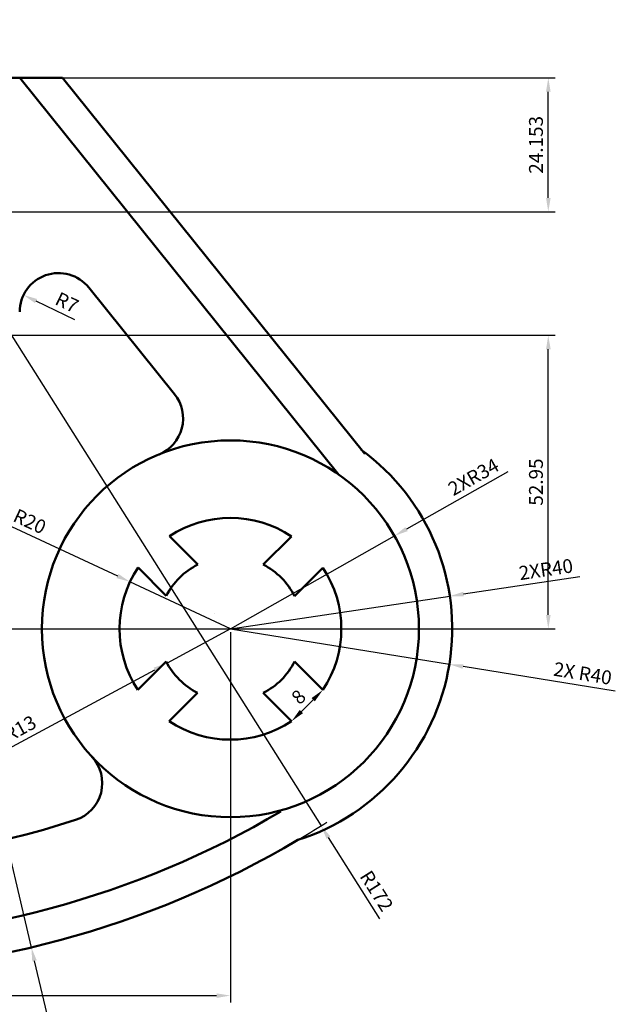
# Model space of a CAD drawing. Units: millimetres. Extents: x 2455 to 2735, y 1365 to 1648.
# Tile 3 of 3: x 2628 to 2735, y 1460 to 1637. Entities that reach past the tile are written whole.
import ezdxf

# ---------------------------------------------------------------- set-up
doc = ezdxf.new("R2010")
doc.units = ezdxf.units.MM
doc.linetypes.add('CENTER', pattern=[50.8, 31.75, -6.35, 6.35, -6.35])
for name, color, linetype, lineweight in [('M-CNTR', 4, 'CENTER', 18), ('M-CONS', 8, 'Continuous', 13), ('M-DIMS', 2, 'Continuous', 25), ('M-OUTL', 7, 'Continuous', 50)]:
    doc.layers.add(name, color=color, linetype=linetype, lineweight=lineweight)
doc.styles.get("Standard").update_dxf_attribs({"font": 'arial.ttf'})
doc.dimstyles.new('ISO-25', dxfattribs={"dimtxt": 2.5, "dimasz": 2.5, "dimexe": 1.25, "dimexo": 0.625, "dimtad": 1, "dimdec": 0, "dimtxsty": 'Standard', "dimcen": 2.5, "dimadec": 0, "dimazin": 0, "dimtfac": 1, "dimtdec": 0, "dimtmove": 0, "dimatfit": 3, "dimfxl": 1, "dimarcsym": 0})

# ---------------------------------------------------------------- blocks, each defined once
blk = doc.blocks.new('*D6')
at = {"layer": 'Defpoints', "color": 0, "transparency": 16777216}
for p in [(2515.88, 1527.3), (2665.87, 1527.3), (2665.87, 1461.12)]:
    blk.add_point(p, dxfattribs=at)
at = {"layer": 'M-DIMS', "color": 0, "lineweight": -2, "transparency": 16777216}
for p, q in [((2515.88, 1526.68), (2515.88, 1459.87)), ((2665.87, 1526.68), (2665.87, 1459.87)), ((2518.38, 1461.12), (2663.37, 1461.12))]:
    blk.add_line(p, q, dxfattribs=at)
at = {"layer": 'M-DIMS', "color": 0, "transparency": 16777216}
for points in [[(2518.38, 1461.53), (2518.38, 1460.7), (2515.88, 1461.12)], [(2663.37, 1461.53), (2663.37, 1460.7), (2665.87, 1461.12)]]:
    blk.add_solid(points, dxfattribs=at)
at = {"layer": 'M-DIMS', "color": 0, "transparency": 16777216, "insert": (2590.87, 1463.02), "char_height": 2.5, "attachment_point": 5}
blk.add_mtext('150', dxfattribs=at)
blk = doc.blocks.new('*D13')
at = {"layer": 'Defpoints', "color": 0, "transparency": 16777216}
for p in [(2628.57, 1587.53), (2634.88, 1584.49)]:
    blk.add_point(p, dxfattribs=at)
at = {"layer": 'M-DIMS', "color": 0, "lineweight": -2, "transparency": 16777216}
blk.add_line((2637.83, 1583.07), (2630.82, 1586.44), dxfattribs=at)
at = {"layer": 'M-DIMS', "color": 0, "transparency": 16777216}
blk.add_solid([(2631, 1586.82), (2630.64, 1586.07), (2628.57, 1587.53)], dxfattribs=at)
at = {"layer": 'M-DIMS', "color": 0, "transparency": 16777216, "insert": (2636.27, 1585.9), "char_height": 2.5, "attachment_point": 5, "rotation": 334.2857}
blk.add_mtext('R7', dxfattribs=at)
blk = doc.blocks.new('*D16')
at = {"layer": 'Defpoints', "color": 0, "transparency": 16777216}
for p in [(2647.76, 1535.78), (2665.88, 1527.3)]:
    blk.add_point(p, dxfattribs=at)
at = {"layer": 'M-DIMS', "color": 0, "lineweight": -2, "transparency": 16777216}
for p, q in [((2625.49, 1546.19), (2645.49, 1536.84)), ((2665.88, 1527.3), (2647.76, 1535.78))]:
    blk.add_line(p, q, dxfattribs=at)
at = {"layer": 'M-DIMS', "color": 0, "transparency": 16777216}
blk.add_solid([(2645.67, 1537.21), (2645.32, 1536.46), (2647.76, 1535.78)], dxfattribs=at)
at = {"layer": 'M-DIMS', "color": 0, "transparency": 16777216, "insert": (2629.56, 1546.39), "char_height": 2.5, "attachment_point": 5, "rotation": 334.9373}
blk.add_mtext('R20', dxfattribs=at)
blk = doc.blocks.new('*D17')
at = {"layer": 'Defpoints', "color": 0, "transparency": 16777216}
for p in [(2665.88, 1527.3), (2654.44, 1521.12)]:
    blk.add_point(p, dxfattribs=at)
at = {"layer": 'M-DIMS', "color": 0, "lineweight": -2, "transparency": 16777216}
for p, q in [((2665.88, 1527.3), (2654.44, 1521.12)), ((2625.82, 1505.64), (2652.24, 1519.93))]:
    blk.add_line(p, q, dxfattribs=at)
at = {"layer": 'M-DIMS', "color": 0, "transparency": 16777216}
blk.add_solid([(2652.04, 1520.3), (2652.44, 1519.56), (2654.44, 1521.12)], dxfattribs=at)
at = {"layer": 'M-DIMS', "color": 0, "transparency": 16777216, "insert": (2628.09, 1509.03), "char_height": 2.5, "attachment_point": 5, "rotation": 28.4115}
blk.add_mtext('R13', dxfattribs=at)
blk = doc.blocks.new('*D20')
at = {"layer": 'Defpoints', "color": 0, "transparency": 16777216}
for p in [(2695.46, 1544.07), (2665.88, 1527.3)]:
    blk.add_point(p, dxfattribs=at)
at = {"layer": 'M-DIMS', "color": 0, "lineweight": -2, "transparency": 16777216}
for p, q in [((2715.88, 1555.64), (2697.63, 1545.3)), ((2665.88, 1527.3), (2695.46, 1544.07))]:
    blk.add_line(p, q, dxfattribs=at)
at = {"layer": 'M-DIMS', "color": 0, "transparency": 16777216}
blk.add_solid([(2697.43, 1545.66), (2697.84, 1544.93), (2695.46, 1544.07)], dxfattribs=at)
at = {"layer": 'M-DIMS', "color": 0, "transparency": 16777216, "insert": (2709.87, 1554.42), "char_height": 2.5, "attachment_point": 5, "rotation": 29.5354}
blk.add_mtext('2XR34', dxfattribs=at)
blk = doc.blocks.new('*D21')
at = {"layer": 'Defpoints', "color": 0, "transparency": 16777216}
for p in [(2705.44, 1533.2), (2665.88, 1527.3)]:
    blk.add_point(p, dxfattribs=at)
at = {"layer": 'M-DIMS', "color": 0, "lineweight": -2, "transparency": 16777216}
for p, q in [((2728.86, 1536.69), (2707.91, 1533.57)), ((2665.88, 1527.3), (2705.44, 1533.2))]:
    blk.add_line(p, q, dxfattribs=at)
at = {"layer": 'M-DIMS', "color": 0, "transparency": 16777216}
blk.add_solid([(2707.85, 1533.98), (2707.97, 1533.15), (2705.44, 1533.2)], dxfattribs=at)
at = {"layer": 'M-DIMS', "color": 0, "transparency": 16777216, "insert": (2722.82, 1537.71), "char_height": 2.5, "attachment_point": 5, "rotation": 8.4728}
blk.add_mtext('2XR40', dxfattribs=at)
blk = doc.blocks.new('*D22')
at = {"layer": 'Defpoints', "color": 0, "transparency": 16777216}
for p in [(2682.56, 1516.28), (2682.56, 1516.28), (2676.9, 1510.62)]:
    blk.add_point(p, dxfattribs=at)
at = {"layer": 'M-DIMS', "color": 0, "lineweight": -2, "transparency": 16777216}
for p, q in [((2682.12, 1516.72), (2681.68, 1517.16)), ((2678.67, 1512.39), (2680.79, 1514.51)), ((2676.46, 1511.06), (2676.02, 1511.5))]:
    blk.add_line(p, q, dxfattribs=at)
at = {"layer": 'M-DIMS', "color": 0, "transparency": 16777216}
for points in [[(2680.5, 1514.8), (2681.09, 1514.21), (2682.56, 1516.28)], [(2678.38, 1512.68), (2678.97, 1512.09), (2676.9, 1510.62)]]:
    blk.add_solid(points, dxfattribs=at)
at = {"layer": 'M-DIMS', "color": 0, "transparency": 16777216, "insert": (2678.39, 1514.79), "char_height": 2.5, "attachment_point": 5, "rotation": 45}
blk.add_mtext('8', dxfattribs=at)
blk = doc.blocks.new('*D23')
at = {"layer": 'Defpoints', "color": 0, "transparency": 16777216}
for p in [(2590.42, 1637.21), (2682.22, 1491.75)]:
    blk.add_point(p, dxfattribs=at)
at = {"layer": 'M-DIMS', "color": 0, "lineweight": -2, "transparency": 16777216}
for p, q in [((2590.42, 1637.21), (2682.22, 1491.75)), ((2692.82, 1474.97), (2683.56, 1489.64))]:
    blk.add_line(p, q, dxfattribs=at)
blk.add_arc((2590.42, 1637.21), 172, 300.8351, 302.6735, dxfattribs=at)
at = {"layer": 'M-DIMS', "color": 0, "transparency": 16777216}
blk.add_solid([(2683.91, 1489.86), (2683.21, 1489.42), (2682.22, 1491.75)], dxfattribs=at)
at = {"layer": 'M-DIMS', "color": 0, "transparency": 16777216, "insert": (2691.97, 1479.84), "char_height": 2.5, "attachment_point": 5, "rotation": 302.2571}
blk.add_mtext('R172', dxfattribs=at)
blk = doc.blocks.new('*D28')
at = {"layer": 'Defpoints', "color": 0, "transparency": 16777216}
for p in [(2570.88, 1580.26), (2723.2, 1580.26), (2515.88, 1527.3)]:
    blk.add_point(p, dxfattribs=at)
at = {"layer": 'M-DIMS', "color": 0, "lineweight": -2, "transparency": 16777216}
for p, q in [((2571.5, 1580.26), (2724.45, 1580.26)), ((2723.2, 1529.8), (2723.2, 1577.76)), ((2516.5, 1527.3), (2724.45, 1527.3))]:
    blk.add_line(p, q, dxfattribs=at)
at = {"layer": 'M-DIMS', "color": 0, "transparency": 16777216}
for points in [[(2722.79, 1577.76), (2723.62, 1577.76), (2723.2, 1580.26)], [(2722.79, 1529.8), (2723.62, 1529.8), (2723.2, 1527.3)]]:
    blk.add_solid(points, dxfattribs=at)
at = {"layer": 'M-DIMS', "color": 0, "transparency": 16777216, "insert": (2721.3, 1553.78), "char_height": 2.5, "attachment_point": 5, "rotation": 90}
blk.add_mtext('52.95', dxfattribs=at)
blk = doc.blocks.new('*D30')
at = {"layer": 'Defpoints', "color": 0, "transparency": 16777216}
for p in [(2566.88, 1626.71), (2723.2, 1626.71), (2572.88, 1602.56)]:
    blk.add_point(p, dxfattribs=at)
at = {"layer": 'M-DIMS', "color": 0, "lineweight": -2, "transparency": 16777216}
for p, q in [((2567.5, 1626.71), (2724.45, 1626.71)), ((2723.2, 1605.06), (2723.2, 1624.21)), ((2573.5, 1602.56), (2724.45, 1602.56))]:
    blk.add_line(p, q, dxfattribs=at)
at = {"layer": 'M-DIMS', "color": 0, "transparency": 16777216}
for points in [[(2722.79, 1624.21), (2723.62, 1624.21), (2723.2, 1626.71)], [(2722.79, 1605.06), (2723.62, 1605.06), (2723.2, 1602.56)]]:
    blk.add_solid(points, dxfattribs=at)
at = {"layer": 'M-DIMS', "color": 0, "transparency": 16777216, "insert": (2721.3, 1614.63), "char_height": 2.5, "attachment_point": 5, "rotation": 90}
blk.add_mtext('24.153', dxfattribs=at)
blk = doc.blocks.new('*D33')
at = {"layer": 'Defpoints', "color": 0, "transparency": 16777216}
for p in [(2665.88, 1527.3), (2705.36, 1520.9)]:
    blk.add_point(p, dxfattribs=at)
at = {"layer": 'M-DIMS', "color": 0, "lineweight": -2, "transparency": 16777216}
for p, q in [((2665.88, 1527.3), (2705.36, 1520.9)), ((2735.28, 1516.05), (2707.83, 1520.5))]:
    blk.add_line(p, q, dxfattribs=at)
at = {"layer": 'M-DIMS', "color": 0, "transparency": 16777216}
blk.add_solid([(2707.89, 1520.91), (2707.76, 1520.09), (2705.36, 1520.9)], dxfattribs=at)
at = {"layer": 'M-DIMS', "color": 0, "transparency": 16777216, "insert": (2729.35, 1518.94), "char_height": 2.5, "attachment_point": 5, "rotation": 350.7883}
blk.add_mtext('2X R40', dxfattribs=at)
blk = doc.blocks.new('*D40')
at = {"layer": 'Defpoints', "color": 0, "transparency": 16777216}
for p in [(2590.42, 1637.21), (2629.97, 1469.82)]:
    blk.add_point(p, dxfattribs=at)
at = {"layer": 'M-DIMS', "color": 0, "lineweight": -2, "transparency": 16777216}
for p, q in [((2590.42, 1637.21), (2629.97, 1469.82)), ((2654.75, 1364.93), (2630.55, 1467.38))]:
    blk.add_line(p, q, dxfattribs=at)
at = {"layer": 'M-DIMS', "color": 0, "transparency": 16777216}
blk.add_solid([(2630.95, 1467.48), (2630.14, 1467.29), (2629.97, 1469.82)], dxfattribs=at)
at = {"layer": 'M-DIMS', "color": 0, "transparency": 16777216, "insert": (2655.53, 1369.81), "char_height": 2.5, "attachment_point": 5, "rotation": 283.2931}
blk.add_mtext('R172', dxfattribs=at)

msp = doc.modelspace()

# ---------------------------------------------------------------- linework, layer by layer
at = {"layer": 'M-CNTR', "ltscale": 0.25, "transparency": 33554534}
msp.add_line((2481.8759, 1527.3043), (2699.8759, 1527.3043), dxfattribs=at)
at = {"layer": 'M-CONS'}
for p, q in [((2663.0522, 1530.1375), (2663.0498, 1530.1351)), ((2660.219, 1527.3138), (2660.2096, 1527.3043)), ((2660.2284, 1527.3043), (2660.219, 1527.3138)), ((2660.2284, 1527.3043), (2660.219, 1527.3138)), ((2660.2284, 1527.3043), (2660.219, 1527.3138)), ((2641.7942, 1503.3029), (2641.692, 1503.2011))]:
    msp.add_line(p, q, dxfattribs=at)
at = {"layer": 'M-OUTL'}
for p, q in [((2614.8759, 1626.7079), (2627.8759, 1626.7079)), ((2685.4509, 1555.1039), (2627.8759, 1626.7079)), ((2627.8759, 1626.7079), (2635.5749, 1626.7079)), ((2690.1268, 1558.8637), (2635.5749, 1626.7079)), ((2655.8016, 1569.6359), (2640.3311, 1588.8761)), ((2659.9772, 1538.889), (2654.8757, 1544.0075)), ((2671.7939, 1538.8792), (2676.9038, 1543.9892)), ((2654.3109, 1533.2416), (2649.2095, 1538.3601)), ((2654.3109, 1533.2416), (2649.2095, 1538.3601)), ((2654.3109, 1533.2416), (2649.2095, 1538.3601)), ((2677.4507, 1533.2223), (2682.5607, 1538.3323)), ((2654.2912, 1521.4057), (2649.1727, 1516.3042)), ((2677.4507, 1521.3863), (2682.5607, 1516.2764)), ((2659.9386, 1515.7394), (2654.8201, 1510.6379)), ((2671.7939, 1515.7295), (2676.9038, 1510.6195))]:
    msp.add_line(p, q, dxfattribs=at)
msp.add_circle((2665.8759, 1527.3043), 34, dxfattribs=at)
for centre, radius, start, end in [((2634.8759, 1584.4896), 7, 38.801949, 180), ((2650.3464, 1565.2495), 7, 292.257336, 38.801949), ((2665.8759, 1527.3043), 40, 287.71708, 53.85854), ((2665.8759, 1527.3043), 20, 56.536959, 123.367439), ((2665.8759, 1527.3043), 13, 116.984185, 152.824611), ((2665.8759, 1527.3043), 13, 27.079787, 62.920213), ((2665.8759, 1527.3043), 20, 146.441357, 213.367439), ((2665.8759, 1527.3043), 20, 326.536959, 33.463041), ((2665.8759, 1527.3043), 13, 206.984185, 242.824611), ((2665.8759, 1527.3043), 13, 297.079787, 332.920213), ((2665.8759, 1527.3043), 20, 236.441357, 303.463041), ((2635.7636, 1499.4789), 7, 288.221236, 42.739702), ((2590.424, 1637.2081), 166, 238.871706, 300.62686), ((2590.424, 1637.2081), 152, 252.066838, 288.221236), ((2590.424, 1637.2081), 172, 238.871706, 300.62686)]:
    msp.add_arc(centre, radius, start, end, dxfattribs=at)

# ---------------------------------------------------------------- dimensions: what is measured, and where the dimension line sits
at = {"layer": 'M-DIMS'}
for center, mpoint, override, picture, middle in [((2590.424, 1637.2081), (2682.2237, 1491.7543), {"dimclrd": 0, "dimclre": 0, "dimclrt": 0}, '*D23', (2690.3772, 1478.8354)), ((2590.424, 1637.2081), (2629.9725, 1469.8165), {"dimdec": 0, "dimlfac": 1, "dimrnd": 0, "dimzin": 0, "dimdsep": 46, "dimlunit": 2}, '*D40', (2653.7015, 1369.3816)), ((2634.8759, 1584.4896), (2628.5691, 1587.5268), {"dimclrd": 0, "dimclre": 0, "dimclrt": 0}, '*D13', (2635.4531, 1584.2117)), ((2665.8759, 1527.3043), (2647.759, 1535.7765), {"dimclrd": 0, "dimclre": 0, "dimclrt": 0}, '*D16', (2628.753, 1544.6645)), ((2665.8759, 1527.3043), (2654.4417, 1521.1189), {"dimclrd": 0, "dimclre": 0, "dimclrt": 0}, '*D17', (2628.9987, 1507.3554))]:
    dim = msp.add_radius_dim(center=center, mpoint=mpoint, dimstyle='ISO-25', override=override, dxfattribs=at)
    dim.commit()
    dim.dimension.update_dxf_attribs({"geometry": picture, "text_midpoint": middle, "dimtype": 164})
for base, p1, p2, override, picture, middle in [((2723.204, 1626.7079), (2572.8759, 1602.555), (2566.8759, 1626.7079), {"dimdec": 3, "dimlfac": 1, "dimrnd": 0, "dimzin": 0, "dimdsep": 46, "dimlunit": 2}, '*D30', (2721.3017, 1614.6315)), ((2723.204, 1580.2571), (2515.8759, 1527.3043), (2570.8759, 1580.2571), {"dimdec": 2, "dimlfac": 1, "dimrnd": 0, "dimzin": 0, "dimdsep": 46, "dimlunit": 2}, '*D28', (2721.3025, 1553.7807))]:
    dim = msp.add_linear_dim(base=base, p1=p1, p2=p2, angle=90, dimstyle='ISO-25', override=override, dxfattribs=at)
    dim.commit()
    dim.dimension.update_dxf_attribs({"geometry": picture, "text_midpoint": middle})
for mpoint, text, override, picture, middle in [((2695.4576, 1544.065), '2X<>', {"dimclrd": 0, "dimclre": 0, "dimclrt": 0}, '*D20', (2710.8117, 1552.7645)), ((2705.4393, 1533.1979), '2X<>', {"dimclrd": 0, "dimclre": 0, "dimclrt": 0}, '*D21', (2723.0959, 1535.8281)), ((2705.36, 1520.901), '2X <>', {"dimdec": 0, "dimlfac": 1, "dimrnd": 0, "dimzin": 0, "dimdsep": 46, "dimlunit": 2}, '*D33', (2729.0505, 1517.059))]:
    dim = msp.add_radius_dim(center=(2665.8759, 1527.3043), mpoint=mpoint, text=text, dimstyle='ISO-25', override=override, dxfattribs=at)
    dim.commit()
    dim.dimension.update_dxf_attribs({"geometry": picture, "text_midpoint": middle, "dimtype": 164})
dim = msp.add_linear_dim(base=(2665.8712, 1461.1167), p1=(2515.8759, 1527.3043), p2=(2665.8712, 1527.3043), dimstyle='ISO-25', override={"dimclrd": 0, "dimclre": 0, "dimclrt": 0}, dxfattribs=at)
dim.commit()
dim.dimension.update_dxf_attribs({"geometry": '*D6', "text_midpoint": (2590.8735, 1463.0182)})
dim = msp.add_aligned_dim(p1=(2676.9038, 1510.6195), p2=(2682.5607, 1516.2764), distance=0, dimstyle='ISO-25', override={"dimclrd": 0, "dimclre": 0, "dimclrt": 0}, dxfattribs=at)
dim.commit()
dim.dimension.update_dxf_attribs({"geometry": '*D22', "text_midpoint": (2678.3878, 1514.7924)})

doc.saveas('drawing.dxf')
